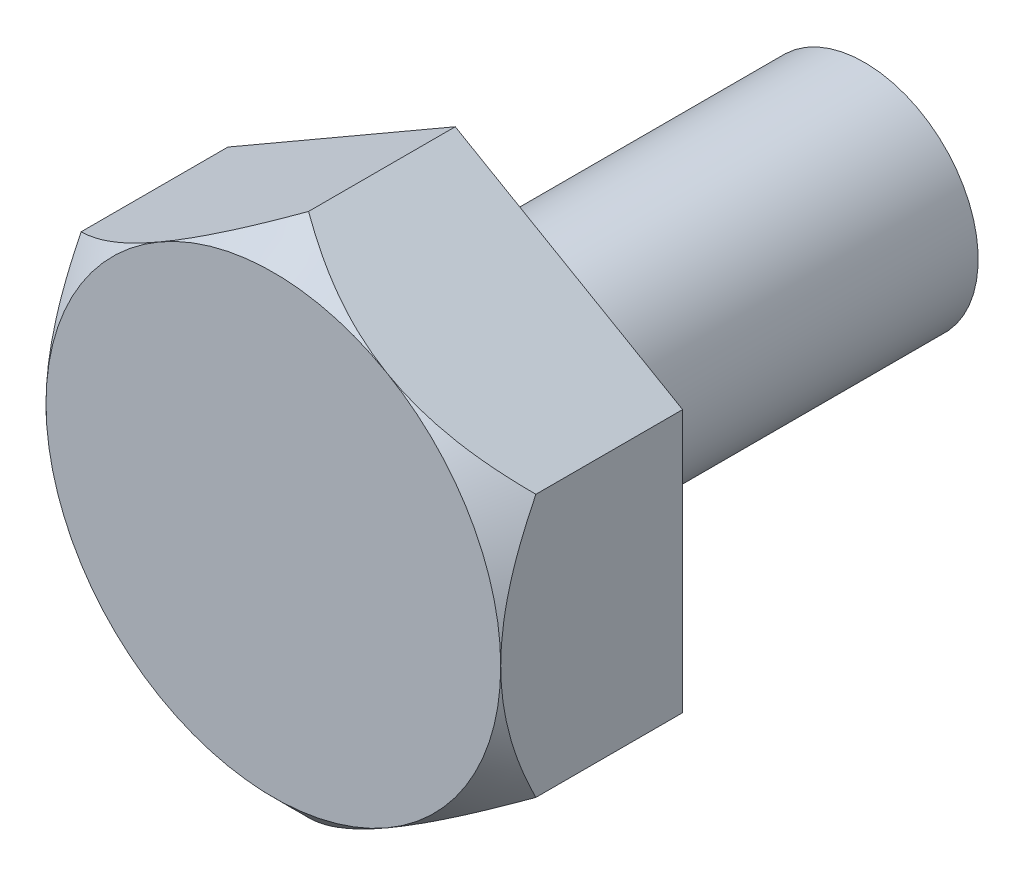
ISO-10303-21;
HEADER;
FILE_DESCRIPTION(('STEP AP214'),'2;1');
FILE_NAME('part.step','',(''),(''),'','','');
FILE_SCHEMA(('AUTOMOTIVE_DESIGN { 1 0 10303 214 1 1 1 1 }'));
ENDSEC;
DATA;
#1=APPLICATION_CONTEXT('core data for automotive mechanical design processes');
#2=APPLICATION_PROTOCOL_DEFINITION('international standard','automotive_design',2000,#1);
#3=PRODUCT_CONTEXT('',#1,'mechanical');
#4=PRODUCT('Part','Part','',(#3));
#5=PRODUCT_RELATED_PRODUCT_CATEGORY('part','',(#4));
#6=PRODUCT_DEFINITION_FORMATION('','',#4);
#7=PRODUCT_DEFINITION_CONTEXT('part definition',#1,'design');
#8=PRODUCT_DEFINITION('design','',#6,#7);
#9=PRODUCT_DEFINITION_SHAPE('','',#8);
#10=(LENGTH_UNIT() NAMED_UNIT(*) SI_UNIT(.MILLI.,.METRE.));
#11=(NAMED_UNIT(*) PLANE_ANGLE_UNIT() SI_UNIT($,.RADIAN.));
#12=(NAMED_UNIT(*) SI_UNIT($,.STERADIAN.) SOLID_ANGLE_UNIT());
#13=UNCERTAINTY_MEASURE_WITH_UNIT(LENGTH_MEASURE(1.E-05),#10,'distance_accuracy_value','');
#14=(GEOMETRIC_REPRESENTATION_CONTEXT(3) GLOBAL_UNCERTAINTY_ASSIGNED_CONTEXT((#13)) GLOBAL_UNIT_ASSIGNED_CONTEXT((#10,
#11,#12)) REPRESENTATION_CONTEXT('',''));
#15=CARTESIAN_POINT('',(0.,0.,0.));
#16=DIRECTION('',(0.,0.,1.));
#17=DIRECTION('',(1.,0.,0.));
#18=AXIS2_PLACEMENT_3D('',#15,#16,#17);
#19=CARTESIAN_POINT('',(0.,-5.77350269189626,4.));
#20=DIRECTION('',(-0.5,0.866025403784439,0.));
#21=DIRECTION('',(-0.866025403784439,-0.5,0.));
#22=AXIS2_PLACEMENT_3D('',#19,#20,#21);
#23=PLANE('',#22);
#24=CARTESIAN_POINT('',(-0.000200000000000018,-5.7736181619501,3.22638183458588));
#25=CARTESIAN_POINT('',(0.0857727681733069,-5.72398176110226,3.27601376249949));
#26=CARTESIAN_POINT('',(0.172406369471809,-5.67396382807171,3.32412258281684));
#27=CARTESIAN_POINT('',(0.347124889028839,-5.57309004377304,3.41683067677397));
#28=CARTESIAN_POINT('',(0.43521056864361,-5.5222337529357,3.46142803360226));
#29=CARTESIAN_POINT('',(0.702658569860331,-5.367822577439,3.58963823597549));
#30=CARTESIAN_POINT('',(0.884284999421829,-5.26296050943972,3.66712224260222));
#31=CARTESIAN_POINT('',(1.25054924277182,-5.05149774994707,3.79980836367823));
#32=CARTESIAN_POINT('',(1.43509343762461,-4.94495110937143,3.85534476745791));
#33=CARTESIAN_POINT('',(1.71494377217238,-4.78337944338747,3.91958681405623));
#34=CARTESIAN_POINT('',(1.8086392399128,-4.72928433986568,3.93781514476511));
#35=CARTESIAN_POINT('',(1.99682352572353,-4.6206360917956,3.96750512097762));
#36=CARTESIAN_POINT('',(2.09131222308105,-4.56608301694086,3.97896777779866));
#37=CARTESIAN_POINT('',(2.32156625980078,-4.43314578685873,3.99818644635776));
#38=CARTESIAN_POINT('',(2.45757968486243,-4.35461839928598,4.00221901984403));
#39=CARTESIAN_POINT('',(2.7293614118944,-4.19770514602325,3.99545145399843));
#40=CARTESIAN_POINT('',(2.86512961123582,-4.11931933958609,3.98464611513274));
#41=CARTESIAN_POINT('',(3.13538603207476,-3.96328672226451,3.9488396582057));
#42=CARTESIAN_POINT('',(3.26987265077585,-3.88564083675503,3.92382266414548));
#43=CARTESIAN_POINT('',(3.53653439939647,-3.73168360440634,3.86095298311431));
#44=CARTESIAN_POINT('',(3.66870970573537,-3.65537215571135,3.82310128033618));
#45=CARTESIAN_POINT('',(3.90334820652232,-3.51990355411976,3.7452274213432));
#46=CARTESIAN_POINT('',(4.0063308906988,-3.4604464736886,3.70725305768472));
#47=CARTESIAN_POINT('',(4.21044753419218,-3.34259967462161,3.62518468192979));
#48=CARTESIAN_POINT('',(4.31158143726392,-3.28420998845894,3.58109048400019));
#49=CARTESIAN_POINT('',(4.51168198823798,-3.16868188148908,3.48777092275138));
#50=CARTESIAN_POINT('',(4.61065432718709,-3.11154017495448,3.43856169539435));
#51=CARTESIAN_POINT('',(4.80676624461305,-2.99831490663731,3.33565818526074));
#52=CARTESIAN_POINT('',(4.90390690306938,-2.94223072132829,3.28196665355472));
#53=CARTESIAN_POINT('',(5.0002,-2.88663587589429,3.22638183458587));
#54=B_SPLINE_CURVE_WITH_KNOTS('',3,(#24,#25,#26,#27,#28,#29,#30,#31,#32,#33,#34,#35,#36,#37,#38,
#39,#40,#41,#42,#43,#44,#45,#46,#47,#48,#49,#50,#51,#52,#53),.UNSPECIFIED.,.F.,.F.,(4,2,2,2,2,2,
2,2,2,2,2,2,2,2,4),(0.,0.332945616209568,0.666071736106991,1.33592065243334,1.99513262597481,
2.32409207808824,2.65300234563691,3.12358963991983,3.59434188052354,4.06562104077027,
4.53686407049611,4.91117956742317,5.2855064331967,5.65868635377115,6.03163889109472),.UNSPECIFIED.);
#55=CARTESIAN_POINT('',(0.,-5.77350269189626,3.22649730810375));
#56=VERTEX_POINT('',#55);
#57=CARTESIAN_POINT('',(2.5,-4.3301270189222,4.));
#58=VERTEX_POINT('',#57);
#59=EDGE_CURVE('E225',#56,#58,#54,.T.);
#60=ORIENTED_EDGE('',*,*,#59,.F.);
#61=DIRECTION('',(0.,0.,-1.));
#62=VECTOR('',#61,1.);
#63=CARTESIAN_POINT('',(0.,-5.77350269189626,4.));
#64=LINE('',#63,#62);
#65=CARTESIAN_POINT('',(0.,-5.77350269189626,0.));
#66=VERTEX_POINT('',#65);
#67=EDGE_CURVE('E223',#56,#66,#64,.T.);
#68=ORIENTED_EDGE('',*,*,#67,.T.);
#69=DIRECTION('',(0.866025403784439,0.5,0.));
#70=VECTOR('',#69,1.);
#71=CARTESIAN_POINT('',(0.,-5.77350269189626,0.));
#72=LINE('',#71,#70);
#73=CARTESIAN_POINT('',(5.,-2.88675134594813,0.));
#74=VERTEX_POINT('',#73);
#75=EDGE_CURVE('E229',#66,#74,#72,.T.);
#76=ORIENTED_EDGE('',*,*,#75,.T.);
#77=DIRECTION('',(0.,0.,-1.));
#78=VECTOR('',#77,1.);
#79=CARTESIAN_POINT('',(5.,-2.88675134594813,4.));
#80=LINE('',#79,#78);
#81=CARTESIAN_POINT('',(5.,-2.88675134594815,3.22649730810375));
#82=VERTEX_POINT('',#81);
#83=EDGE_CURVE('E246',#82,#74,#80,.T.);
#84=ORIENTED_EDGE('',*,*,#83,.F.);
#85=EDGE_CURVE('E180',#58,#82,#54,.T.);
#86=ORIENTED_EDGE('',*,*,#85,.F.);
#87=EDGE_LOOP('',(#60,#68,#76,#84,#86));
#88=FACE_BOUND('',#87,.T.);
#89=ADVANCED_FACE('F45',(#88),#23,.F.);
#90=CARTESIAN_POINT('',(5.,-2.88675134594813,4.));
#91=DIRECTION('',(-1.,0.,0.));
#92=DIRECTION('',(0.,-1.,0.));
#93=AXIS2_PLACEMENT_3D('',#90,#91,#92);
#94=PLANE('',#93);
#95=CARTESIAN_POINT('',(5.,-9.91072051451662,-2.10055769395665));
#96=CARTESIAN_POINT('',(5.,-9.76621544127602,-1.97154454329479));
#97=CARTESIAN_POINT('',(5.,-9.62142904059379,-1.84284651390385));
#98=CARTESIAN_POINT('',(5.,-9.33121648801016,-1.58617055483695));
#99=CARTESIAN_POINT('',(5.,-9.18579032871603,-1.45819263352135));
#100=CARTESIAN_POINT('',(5.,-8.74834130441583,-1.07539053167285));
#101=CARTESIAN_POINT('',(5.,-8.45524720366472,-0.821786895816466));
#102=CARTESIAN_POINT('',(5.,-7.86187287101059,-0.315830598049089));
#103=CARTESIAN_POINT('',(5.,-7.56154861188113,-0.0635294286387808));
#104=CARTESIAN_POINT('',(5.,-6.95607062007869,0.435107261094935));
#105=CARTESIAN_POINT('',(5.,-6.65091784334251,0.681443938411082));
#106=CARTESIAN_POINT('',(5.,-6.05281956409636,1.15115601537285));
#107=CARTESIAN_POINT('',(5.,-5.76025864959821,1.37501719326704));
#108=CARTESIAN_POINT('',(5.,-5.3155611070372,1.70306559777502));
#109=CARTESIAN_POINT('',(5.,-5.1663052656364,1.81115689472442));
#110=CARTESIAN_POINT('',(5.,-4.86554936597768,2.02416494614329));
#111=CARTESIAN_POINT('',(5.,-4.71404941939871,2.12908185780219));
#112=CARTESIAN_POINT('',(5.,-4.40884314645316,2.33477509223266));
#113=CARTESIAN_POINT('',(5.,-4.25514378185362,2.43556171139529));
#114=CARTESIAN_POINT('',(5.,-3.94471151466891,2.63239951344171));
#115=CARTESIAN_POINT('',(5.,-3.78797837092588,2.72845031770066));
#116=CARTESIAN_POINT('',(5.,-3.47117914660732,2.91455296566001));
#117=CARTESIAN_POINT('',(5.,-3.31111650469861,3.00461063098044));
#118=CARTESIAN_POINT('',(5.,-2.98705558910371,3.17731119527027));
#119=CARTESIAN_POINT('',(5.,-2.82305823727669,3.25995580994437));
#120=CARTESIAN_POINT('',(5.,-2.50246960746522,3.41038679829273));
#121=CARTESIAN_POINT('',(5.,-2.34618024242307,3.47881169830795));
#122=CARTESIAN_POINT('',(5.,-2.02957491141866,3.60572985215042));
#123=CARTESIAN_POINT('',(5.,-1.86925893812462,3.66422308789225));
#124=CARTESIAN_POINT('',(5.,-1.54540593636024,3.76885041954304));
#125=CARTESIAN_POINT('',(5.,-1.38188714698498,3.81504020516505));
#126=CARTESIAN_POINT('',(5.,-1.05149027309675,3.89315112780065));
#127=CARTESIAN_POINT('',(5.,-0.884613565388637,3.9250779931138));
#128=CARTESIAN_POINT('',(5.,-0.545836980273731,3.97313093477257));
#129=CARTESIAN_POINT('',(5.,-0.373899433698271,3.98899706157323));
#130=CARTESIAN_POINT('',(5.,-0.0293097036115672,4.00287735940177));
#131=CARTESIAN_POINT('',(5.,0.143342399655701,4.00089348335961));
#132=CARTESIAN_POINT('',(5.,0.487882402140031,3.97920409445634));
#133=CARTESIAN_POINT('',(5.,0.659767847142363,3.95946033548157));
#134=CARTESIAN_POINT('',(5.,1.00084509884113,3.90359558221986));
#135=CARTESIAN_POINT('',(5.,1.17003611690969,3.86746988111293));
#136=CARTESIAN_POINT('',(5.,1.55360689626622,3.7683614441394));
#137=CARTESIAN_POINT('',(5.,1.76674581305401,3.70061559776904));
#138=CARTESIAN_POINT('',(5.,2.18611598773547,3.54647241114183));
#139=CARTESIAN_POINT('',(5.,2.39234343170509,3.4600649625223));
#140=CARTESIAN_POINT('',(5.,2.80040314281745,3.27207752711923));
#141=CARTESIAN_POINT('',(5.,3.00216331747143,3.17034289977823));
#142=CARTESIAN_POINT('',(5.,3.30029802660671,3.00959150256192));
#143=CARTESIAN_POINT('',(5.,3.39891511024584,2.9546557234027));
#144=CARTESIAN_POINT('',(5.,3.59478493952169,2.84240035369005));
#145=CARTESIAN_POINT('',(5.,3.69203769266294,2.78508077625563));
#146=CARTESIAN_POINT('',(5.,3.93268621485032,2.63974614813006));
#147=CARTESIAN_POINT('',(5.,4.07531703883476,2.55046551491085));
#148=CARTESIAN_POINT('',(5.,4.35814665684457,2.36812363187614));
#149=CARTESIAN_POINT('',(5.,4.49834523281012,2.27506204555858));
#150=CARTESIAN_POINT('',(5.,4.91585745402423,1.9911616420883));
#151=CARTESIAN_POINT('',(5.,5.19000092006772,1.79566062403075));
#152=CARTESIAN_POINT('',(5.,5.7323797860828,1.39561219564106));
#153=CARTESIAN_POINT('',(5.,6.00060231013792,1.19104751794871));
#154=CARTESIAN_POINT('',(5.,6.53211217027,0.775583147109073));
#155=CARTESIAN_POINT('',(5.,6.79539913149934,0.564682975932098));
#156=CARTESIAN_POINT('',(5.,7.30031300079127,0.15269603485646));
#157=CARTESIAN_POINT('',(5.,7.542193814675,-0.0480807930482146));
#158=CARTESIAN_POINT('',(5.,8.02327968337917,-0.452837162951994));
#159=CARTESIAN_POINT('',(5.,8.26248458717145,-0.656816884175983));
#160=CARTESIAN_POINT('',(5.,8.73754753272066,-1.06629372433063));
#161=CARTESIAN_POINT('',(5.,8.97341623310163,-1.27177850235316));
#162=CARTESIAN_POINT('',(5.,9.44333428124391,-1.68476461510824));
#163=CARTESIAN_POINT('',(5.,9.67738383656504,-1.89226571351926));
#164=CARTESIAN_POINT('',(5.,9.91072051451663,-2.10055769395665));
#165=B_SPLINE_CURVE_WITH_KNOTS('',3,(#95,#96,#97,#98,#99,#100,#101,#102,#103,#104,#105,#106,
#107,#108,#109,#110,#111,#112,#113,#114,#115,#116,#117,#118,#119,#120,#121,#122,#123,#124,#125,
#126,#127,#128,#129,#130,#131,#132,#133,#134,#135,#136,#137,#138,#139,#140,#141,#142,#143,#144,
#145,#146,#147,#148,#149,#150,#151,#152,#153,#154,#155,#156,#157,#158,#159,#160,#161,#162,#163,
#164),.UNSPECIFIED.,.F.,.F.,(4,2,2,2,2,2,2,2,2,2,2,2,2,2,2,2,2,2,2,2,2,2,2,2,2,2,2,2,2,2,2,2,2,
2,4),(0.,0.581148909212411,1.16230455163196,2.32501564731192,3.50167323602094,4.67810071770477,
5.78306048880437,6.33588410810416,6.88868030769224,7.44000224568793,7.99136819022149,
8.5421904855475,9.09288496573265,9.6044443239522,10.1160046137044,10.6252084636211,
11.1342076219167,11.6513194059097,12.1683746145159,12.6865459803083,13.2048663202667,
13.8746333370564,14.5447640581128,15.2221753046931,15.5608090570693,15.8994409460531,
16.4041719839859,16.9089480414397,17.9188053190632,18.9306770062131,19.9426252344689,
20.8856511270215,21.8287299780402,22.7671855689286,23.7055324644857),.UNSPECIFIED.);
#166=CARTESIAN_POINT('',(5.,0.,4.));
#167=VERTEX_POINT('',#166);
#168=EDGE_CURVE('E271',#82,#167,#165,.T.);
#169=ORIENTED_EDGE('',*,*,#168,.F.);
#170=ORIENTED_EDGE('',*,*,#83,.T.);
#171=DIRECTION('',(0.,1.,0.));
#172=VECTOR('',#171,1.);
#173=CARTESIAN_POINT('',(5.,-2.88675134594813,0.));
#174=LINE('',#173,#172);
#175=CARTESIAN_POINT('',(5.,2.88675134594813,0.));
#176=VERTEX_POINT('',#175);
#177=EDGE_CURVE('E266',#74,#176,#174,.T.);
#178=ORIENTED_EDGE('',*,*,#177,.T.);
#179=DIRECTION('',(0.,0.,-1.));
#180=VECTOR('',#179,1.);
#181=CARTESIAN_POINT('',(5.,2.88675134594813,4.));
#182=LINE('',#181,#180);
#183=CARTESIAN_POINT('',(5.,2.88675134594813,3.22649730810375));
#184=VERTEX_POINT('',#183);
#185=EDGE_CURVE('E245',#184,#176,#182,.T.);
#186=ORIENTED_EDGE('',*,*,#185,.F.);
#187=EDGE_CURVE('E118',#167,#184,#165,.T.);
#188=ORIENTED_EDGE('',*,*,#187,.F.);
#189=EDGE_LOOP('',(#169,#170,#178,#186,#188));
#190=FACE_BOUND('',#189,.T.);
#191=ADVANCED_FACE('F213',(#190),#94,.F.);
#192=CARTESIAN_POINT('',(5.,2.88675134594813,4.));
#193=DIRECTION('',(-0.5,-0.866025403784439,0.));
#194=DIRECTION('',(0.866025403784439,-0.5,0.));
#195=AXIS2_PLACEMENT_3D('',#192,#193,#194);
#196=PLANE('',#195);
#197=CARTESIAN_POINT('',(5.0002,2.88663587589429,3.22638183458588));
#198=CARTESIAN_POINT('',(4.91422723182669,2.93627227674213,3.27601376249948));
#199=CARTESIAN_POINT('',(4.82759363052819,2.98629020977269,3.32412258281684));
#200=CARTESIAN_POINT('',(4.65287511097116,3.08716399407135,3.41683067677397));
#201=CARTESIAN_POINT('',(4.56478943135639,3.13802028490869,3.46142803360226));
#202=CARTESIAN_POINT('',(4.29734143013967,3.29243146040539,3.58963823597549));
#203=CARTESIAN_POINT('',(4.11571500057817,3.39729352840467,3.66712224260222));
#204=CARTESIAN_POINT('',(3.74945075722818,3.60875628789733,3.79980836367823));
#205=CARTESIAN_POINT('',(3.56490656237539,3.71530292847296,3.85534476745791));
#206=CARTESIAN_POINT('',(3.28505622782762,3.87687459445692,3.91958681405623));
#207=CARTESIAN_POINT('',(3.1913607600872,3.93096969797871,3.93781514476511));
#208=CARTESIAN_POINT('',(3.00317647427647,4.03961794604879,3.96750512097762));
#209=CARTESIAN_POINT('',(2.90868777691895,4.09417102090353,3.97896777779866));
#210=CARTESIAN_POINT('',(2.67843374019922,4.22710825098566,3.99818644635776));
#211=CARTESIAN_POINT('',(2.54242031513757,4.30563563855841,4.00221901984403));
#212=CARTESIAN_POINT('',(2.2706385881056,4.46254889182114,3.99545145399843));
#213=CARTESIAN_POINT('',(2.13487038876418,4.5409346982583,3.98464611513274));
#214=CARTESIAN_POINT('',(1.86461396792524,4.69696731557988,3.9488396582057));
#215=CARTESIAN_POINT('',(1.73012734922416,4.77461320108936,3.92382266414548));
#216=CARTESIAN_POINT('',(1.46346560060354,4.92857043343805,3.86095298311431));
#217=CARTESIAN_POINT('',(1.33129029426463,5.00488188213304,3.82310128033618));
#218=CARTESIAN_POINT('',(1.09665179347769,5.14035048372463,3.7452274213432));
#219=CARTESIAN_POINT('',(0.993669109301204,5.19980756415579,3.70725305768472));
#220=CARTESIAN_POINT('',(0.789552465807829,5.31765436322278,3.62518468192979));
#221=CARTESIAN_POINT('',(0.688418562736081,5.37604404938545,3.58109048400019));
#222=CARTESIAN_POINT('',(0.488318011762026,5.49157215635531,3.48777092275138));
#223=CARTESIAN_POINT('',(0.38934567281291,5.54871386288991,3.43856169539435));
#224=CARTESIAN_POINT('',(0.193233755386958,5.66193913120708,3.33565818526074));
#225=CARTESIAN_POINT('',(0.0960930969306188,5.7180233165161,3.28196665355472));
#226=CARTESIAN_POINT('',(-0.000199999999999045,5.7736181619501,3.22638183458588));
#227=B_SPLINE_CURVE_WITH_KNOTS('',3,(#197,#198,#199,#200,#201,#202,#203,#204,#205,#206,#207,
#208,#209,#210,#211,#212,#213,#214,#215,#216,#217,#218,#219,#220,#221,#222,#223,#224,#225,#226),
.UNSPECIFIED.,.F.,.F.,(4,2,2,2,2,2,2,2,2,2,2,2,2,2,4),(0.,0.332945616209569,0.666071736106991,
1.33592065243334,1.99513262597481,2.32409207808824,2.65300234563691,3.12358963991983,
3.59434188052354,4.06562104077027,4.53686407049611,4.91117956742317,5.2855064331967,
5.65868635377115,6.03163889109472),.UNSPECIFIED.);
#228=CARTESIAN_POINT('',(2.5,4.3301270189222,4.));
#229=VERTEX_POINT('',#228);
#230=EDGE_CURVE('E113',#184,#229,#227,.T.);
#231=ORIENTED_EDGE('',*,*,#230,.F.);
#232=ORIENTED_EDGE('',*,*,#185,.T.);
#233=DIRECTION('',(-0.866025403784439,0.5,0.));
#234=VECTOR('',#233,1.);
#235=CARTESIAN_POINT('',(5.,2.88675134594813,0.));
#236=LINE('',#235,#234);
#237=CARTESIAN_POINT('',(0.,5.77350269189626,0.));
#238=VERTEX_POINT('',#237);
#239=EDGE_CURVE('E270',#176,#238,#236,.T.);
#240=ORIENTED_EDGE('',*,*,#239,.T.);
#241=DIRECTION('',(0.,0.,-1.));
#242=VECTOR('',#241,1.);
#243=CARTESIAN_POINT('',(0.,5.77350269189626,4.));
#244=LINE('',#243,#242);
#245=CARTESIAN_POINT('',(0.,5.77350269189626,3.22649730810375));
#246=VERTEX_POINT('',#245);
#247=EDGE_CURVE('E142',#246,#238,#244,.T.);
#248=ORIENTED_EDGE('',*,*,#247,.F.);
#249=EDGE_CURVE('E122',#229,#246,#227,.T.);
#250=ORIENTED_EDGE('',*,*,#249,.F.);
#251=EDGE_LOOP('',(#231,#232,#240,#248,#250));
#252=FACE_BOUND('',#251,.T.);
#253=ADVANCED_FACE('F139',(#252),#196,.F.);
#254=CARTESIAN_POINT('',(0.,5.77350269189626,4.));
#255=DIRECTION('',(0.5,-0.866025403784439,0.));
#256=DIRECTION('',(0.866025403784439,0.5,0.));
#257=AXIS2_PLACEMENT_3D('',#254,#255,#256);
#258=PLANE('',#257);
#259=CARTESIAN_POINT('',(0.000200000000001333,5.7736181619501,3.22638183458588));
#260=CARTESIAN_POINT('',(-0.085772768173306,5.72398176110226,3.27601376249948));
#261=CARTESIAN_POINT('',(-0.172406369471808,5.67396382807171,3.32412258281684));
#262=CARTESIAN_POINT('',(-0.347124889028838,5.57309004377304,3.41683067677397));
#263=CARTESIAN_POINT('',(-0.435210568643609,5.5222337529357,3.46142803360226));
#264=CARTESIAN_POINT('',(-0.70265856986033,5.367822577439,3.58963823597549));
#265=CARTESIAN_POINT('',(-0.884284999421829,5.26296050943972,3.66712224260222));
#266=CARTESIAN_POINT('',(-1.25054924277182,5.05149774994706,3.79980836367823));
#267=CARTESIAN_POINT('',(-1.43509343762461,4.94495110937143,3.85534476745791));
#268=CARTESIAN_POINT('',(-1.71494377217238,4.78337944338747,3.91958681405623));
#269=CARTESIAN_POINT('',(-1.8086392399128,4.72928433986569,3.93781514476511));
#270=CARTESIAN_POINT('',(-1.99682352572353,4.6206360917956,3.96750512097762));
#271=CARTESIAN_POINT('',(-2.09131222308105,4.56608301694086,3.97896777779866));
#272=CARTESIAN_POINT('',(-2.32156625980078,4.43314578685873,3.99818644635776));
#273=CARTESIAN_POINT('',(-2.45757968486243,4.35461839928598,4.00221901984403));
#274=CARTESIAN_POINT('',(-2.7293614118944,4.19770514602325,3.99545145399843));
#275=CARTESIAN_POINT('',(-2.86512961123582,4.11931933958609,3.98464611513274));
#276=CARTESIAN_POINT('',(-3.13538603207476,3.96328672226451,3.9488396582057));
#277=CARTESIAN_POINT('',(-3.26987265077584,3.88564083675503,3.92382266414548));
#278=CARTESIAN_POINT('',(-3.53653439939646,3.73168360440634,3.86095298311431));
#279=CARTESIAN_POINT('',(-3.66870970573537,3.65537215571135,3.82310128033618));
#280=CARTESIAN_POINT('',(-3.90334820652231,3.51990355411976,3.7452274213432));
#281=CARTESIAN_POINT('',(-4.0063308906988,3.4604464736886,3.70725305768472));
#282=CARTESIAN_POINT('',(-4.21044753419217,3.34259967462161,3.6251846819298));
#283=CARTESIAN_POINT('',(-4.31158143726392,3.28420998845894,3.58109048400019));
#284=CARTESIAN_POINT('',(-4.51168198823798,3.16868188148908,3.48777092275138));
#285=CARTESIAN_POINT('',(-4.61065432718709,3.11154017495448,3.43856169539435));
#286=CARTESIAN_POINT('',(-4.80676624461304,2.99831490663731,3.33565818526074));
#287=CARTESIAN_POINT('',(-4.90390690306938,2.94223072132829,3.28196665355473));
#288=CARTESIAN_POINT('',(-5.0002,2.88663587589429,3.22638183458588));
#289=B_SPLINE_CURVE_WITH_KNOTS('',3,(#259,#260,#261,#262,#263,#264,#265,#266,#267,#268,#269,
#270,#271,#272,#273,#274,#275,#276,#277,#278,#279,#280,#281,#282,#283,#284,#285,#286,#287,#288),
.UNSPECIFIED.,.F.,.F.,(4,2,2,2,2,2,2,2,2,2,2,2,2,2,4),(0.,0.332945616209568,0.666071736106991,
1.33592065243334,1.99513262597481,2.32409207808824,2.65300234563691,3.12358963991983,
3.59434188052353,4.06562104077027,4.53686407049611,4.91117956742317,5.2855064331967,
5.65868635377115,6.03163889109472),.UNSPECIFIED.);
#290=CARTESIAN_POINT('',(-2.5,4.3301270189222,4.));
#291=VERTEX_POINT('',#290);
#292=EDGE_CURVE('E129',#246,#291,#289,.T.);
#293=ORIENTED_EDGE('',*,*,#292,.F.);
#294=ORIENTED_EDGE('',*,*,#247,.T.);
#295=DIRECTION('',(-0.866025403784439,-0.5,0.));
#296=VECTOR('',#295,1.);
#297=CARTESIAN_POINT('',(0.,5.77350269189626,0.));
#298=LINE('',#297,#296);
#299=CARTESIAN_POINT('',(-5.,2.88675134594813,0.));
#300=VERTEX_POINT('',#299);
#301=EDGE_CURVE('E263',#238,#300,#298,.T.);
#302=ORIENTED_EDGE('',*,*,#301,.T.);
#303=DIRECTION('',(0.,0.,-1.));
#304=VECTOR('',#303,1.);
#305=CARTESIAN_POINT('',(-5.,2.88675134594813,4.));
#306=LINE('',#305,#304);
#307=CARTESIAN_POINT('',(-5.,2.88675134594815,3.22649730810375));
#308=VERTEX_POINT('',#307);
#309=EDGE_CURVE('E240',#308,#300,#306,.T.);
#310=ORIENTED_EDGE('',*,*,#309,.F.);
#311=EDGE_CURVE('E141',#291,#308,#289,.T.);
#312=ORIENTED_EDGE('',*,*,#311,.F.);
#313=EDGE_LOOP('',(#293,#294,#302,#310,#312));
#314=FACE_BOUND('',#313,.T.);
#315=ADVANCED_FACE('F204',(#314),#258,.F.);
#316=CARTESIAN_POINT('',(-5.,2.88675134594813,4.));
#317=DIRECTION('',(1.,0.,0.));
#318=DIRECTION('',(0.,0.,-1.));
#319=AXIS2_PLACEMENT_3D('',#316,#317,#318);
#320=PLANE('',#319);
#321=CARTESIAN_POINT('',(-5.,9.91072051451663,-2.10055769395665));
#322=CARTESIAN_POINT('',(-5.,9.76621544127602,-1.97154454329479));
#323=CARTESIAN_POINT('',(-5.,9.62142904059379,-1.84284651390385));
#324=CARTESIAN_POINT('',(-5.,9.33121648801016,-1.58617055483695));
#325=CARTESIAN_POINT('',(-5.,9.18579032871603,-1.45819263352135));
#326=CARTESIAN_POINT('',(-5.,8.74834130441583,-1.07539053167285));
#327=CARTESIAN_POINT('',(-5.,8.45524720366472,-0.821786895816467));
#328=CARTESIAN_POINT('',(-5.,7.86187287101059,-0.315830598049089));
#329=CARTESIAN_POINT('',(-5.,7.56154861188114,-0.0635294286387806));
#330=CARTESIAN_POINT('',(-5.,6.95607062007869,0.435107261094936));
#331=CARTESIAN_POINT('',(-5.,6.65091784334251,0.681443938411084));
#332=CARTESIAN_POINT('',(-5.,6.05281956409636,1.15115601537285));
#333=CARTESIAN_POINT('',(-5.,5.76025864959822,1.37501719326704));
#334=CARTESIAN_POINT('',(-5.,5.3155611070372,1.70306559777502));
#335=CARTESIAN_POINT('',(-5.,5.1663052656364,1.81115689472442));
#336=CARTESIAN_POINT('',(-5.,4.86554936597768,2.02416494614329));
#337=CARTESIAN_POINT('',(-5.,4.71404941939871,2.12908185780219));
#338=CARTESIAN_POINT('',(-5.,4.40884314645316,2.33477509223266));
#339=CARTESIAN_POINT('',(-5.,4.25514378185362,2.43556171139529));
#340=CARTESIAN_POINT('',(-5.,3.94471151466891,2.63239951344171));
#341=CARTESIAN_POINT('',(-5.,3.78797837092588,2.72845031770066));
#342=CARTESIAN_POINT('',(-5.,3.47117914660733,2.91455296566001));
#343=CARTESIAN_POINT('',(-5.,3.31111650469862,3.00461063098044));
#344=CARTESIAN_POINT('',(-5.,2.98705558910371,3.17731119527027));
#345=CARTESIAN_POINT('',(-5.,2.82305823727669,3.25995580994437));
#346=CARTESIAN_POINT('',(-5.,2.50246960746522,3.41038679829273));
#347=CARTESIAN_POINT('',(-5.,2.34618024242307,3.47881169830795));
#348=CARTESIAN_POINT('',(-5.,2.02957491141867,3.60572985215042));
#349=CARTESIAN_POINT('',(-5.,1.86925893812462,3.66422308789225));
#350=CARTESIAN_POINT('',(-5.,1.54540593636025,3.76885041954304));
#351=CARTESIAN_POINT('',(-5.,1.38188714698499,3.81504020516505));
#352=CARTESIAN_POINT('',(-5.,1.05149027309676,3.89315112780065));
#353=CARTESIAN_POINT('',(-5.,0.884613565388641,3.9250779931138));
#354=CARTESIAN_POINT('',(-5.,0.545836980273738,3.97313093477257));
#355=CARTESIAN_POINT('',(-5.,0.373899433698277,3.98899706157323));
#356=CARTESIAN_POINT('',(-5.,0.0293097036115736,4.00287735940177));
#357=CARTESIAN_POINT('',(-5.,-0.143342399655695,4.00089348335961));
#358=CARTESIAN_POINT('',(-5.,-0.487882402140026,3.97920409445635));
#359=CARTESIAN_POINT('',(-5.,-0.659767847142358,3.95946033548157));
#360=CARTESIAN_POINT('',(-5.,-1.00084509884112,3.90359558221986));
#361=CARTESIAN_POINT('',(-5.,-1.17003611690968,3.86746988111293));
#362=CARTESIAN_POINT('',(-5.,-1.55360689626622,3.7683614441394));
#363=CARTESIAN_POINT('',(-5.,-1.76674581305401,3.70061559776904));
#364=CARTESIAN_POINT('',(-5.,-2.18611598773546,3.54647241114183));
#365=CARTESIAN_POINT('',(-5.,-2.39234343170509,3.4600649625223));
#366=CARTESIAN_POINT('',(-5.,-2.80040314281745,3.27207752711923));
#367=CARTESIAN_POINT('',(-5.,-3.00216331747142,3.17034289977824));
#368=CARTESIAN_POINT('',(-5.,-3.3002980266067,3.00959150256193));
#369=CARTESIAN_POINT('',(-5.,-3.39891511024583,2.95465572340271));
#370=CARTESIAN_POINT('',(-5.,-3.59478493952168,2.84240035369006));
#371=CARTESIAN_POINT('',(-5.,-3.69203769266292,2.78508077625564));
#372=CARTESIAN_POINT('',(-5.,-3.93268621485031,2.63974614813007));
#373=CARTESIAN_POINT('',(-5.,-4.07531703883475,2.55046551491086));
#374=CARTESIAN_POINT('',(-5.,-4.35814665684456,2.36812363187615));
#375=CARTESIAN_POINT('',(-5.,-4.49834523281012,2.27506204555858));
#376=CARTESIAN_POINT('',(-5.,-4.91585745402422,1.99116164208831));
#377=CARTESIAN_POINT('',(-5.,-5.19000092006771,1.79566062403075));
#378=CARTESIAN_POINT('',(-5.,-5.7323797860828,1.39561219564107));
#379=CARTESIAN_POINT('',(-5.,-6.00060231013791,1.19104751794872));
#380=CARTESIAN_POINT('',(-5.,-6.53211217027,0.775583147109079));
#381=CARTESIAN_POINT('',(-5.,-6.79539913149933,0.564682975932104));
#382=CARTESIAN_POINT('',(-5.,-7.30031300079127,0.152696034856465));
#383=CARTESIAN_POINT('',(-5.,-7.542193814675,-0.0480807930482094));
#384=CARTESIAN_POINT('',(-5.,-8.02327968337917,-0.452837162951989));
#385=CARTESIAN_POINT('',(-5.,-8.26248458717144,-0.65681688417598));
#386=CARTESIAN_POINT('',(-5.,-8.73754753272065,-1.06629372433062));
#387=CARTESIAN_POINT('',(-5.,-8.97341623310163,-1.27177850235316));
#388=CARTESIAN_POINT('',(-5.,-9.44333428124391,-1.68476461510824));
#389=CARTESIAN_POINT('',(-5.,-9.67738383656504,-1.89226571351926));
#390=CARTESIAN_POINT('',(-5.,-9.91072051451662,-2.10055769395665));
#391=B_SPLINE_CURVE_WITH_KNOTS('',3,(#321,#322,#323,#324,#325,#326,#327,#328,#329,#330,#331,
#332,#333,#334,#335,#336,#337,#338,#339,#340,#341,#342,#343,#344,#345,#346,#347,#348,#349,#350,
#351,#352,#353,#354,#355,#356,#357,#358,#359,#360,#361,#362,#363,#364,#365,#366,#367,#368,#369,
#370,#371,#372,#373,#374,#375,#376,#377,#378,#379,#380,#381,#382,#383,#384,#385,#386,#387,#388,
#389,#390),.UNSPECIFIED.,.F.,.F.,(4,2,2,2,2,2,2,2,2,2,2,2,2,2,2,2,2,2,2,2,2,2,2,2,2,2,2,2,2,2,2,
2,2,2,4),(0.,0.581148909212412,1.16230455163196,2.32501564731192,3.50167323602094,
4.67810071770477,5.78306048880437,6.33588410810416,6.88868030769224,7.44000224568794,
7.99136819022149,8.5421904855475,9.09288496573265,9.6044443239522,10.1160046137044,
10.6252084636211,11.1342076219167,11.6513194059097,12.1683746145159,12.6865459803083,
13.2048663202667,13.8746333370564,14.5447640581128,15.2221753046931,15.5608090570693,
15.8994409460531,16.4041719839859,16.9089480414397,17.9188053190632,18.9306770062131,
19.9426252344689,20.8856511270215,21.8287299780402,22.7671855689286,23.7055324644857),.UNSPECIFIED.);
#392=CARTESIAN_POINT('',(-5.,0.,4.));
#393=VERTEX_POINT('',#392);
#394=EDGE_CURVE('E196',#308,#393,#391,.T.);
#395=ORIENTED_EDGE('',*,*,#394,.F.);
#396=ORIENTED_EDGE('',*,*,#309,.T.);
#397=DIRECTION('',(0.,-1.,0.));
#398=VECTOR('',#397,1.);
#399=CARTESIAN_POINT('',(-5.,2.88675134594813,0.));
#400=LINE('',#399,#398);
#401=CARTESIAN_POINT('',(-5.,-2.88675134594813,0.));
#402=VERTEX_POINT('',#401);
#403=EDGE_CURVE('E239',#300,#402,#400,.T.);
#404=ORIENTED_EDGE('',*,*,#403,.T.);
#405=DIRECTION('',(0.,0.,-1.));
#406=VECTOR('',#405,1.);
#407=CARTESIAN_POINT('',(-5.,-2.88675134594813,4.));
#408=LINE('',#407,#406);
#409=CARTESIAN_POINT('',(-5.,-2.88675134594813,3.22649730810375));
#410=VERTEX_POINT('',#409);
#411=EDGE_CURVE('E234',#410,#402,#408,.T.);
#412=ORIENTED_EDGE('',*,*,#411,.F.);
#413=EDGE_CURVE('E195',#393,#410,#391,.T.);
#414=ORIENTED_EDGE('',*,*,#413,.F.);
#415=EDGE_LOOP('',(#395,#396,#404,#412,#414));
#416=FACE_BOUND('',#415,.T.);
#417=ADVANCED_FACE('F199',(#416),#320,.F.);
#418=CARTESIAN_POINT('',(-5.,-2.88675134594813,4.));
#419=DIRECTION('',(0.5,0.866025403784439,0.));
#420=DIRECTION('',(-0.866025403784439,0.5,0.));
#421=AXIS2_PLACEMENT_3D('',#418,#419,#420);
#422=PLANE('',#421);
#423=CARTESIAN_POINT('',(-5.0002,-2.88663587589429,3.22638183458588));
#424=CARTESIAN_POINT('',(-4.91422723182669,-2.93627227674213,3.27601376249949));
#425=CARTESIAN_POINT('',(-4.82759363052819,-2.98629020977269,3.32412258281684));
#426=CARTESIAN_POINT('',(-4.65287511097116,-3.08716399407135,3.41683067677397));
#427=CARTESIAN_POINT('',(-4.56478943135639,-3.13802028490869,3.46142803360226));
#428=CARTESIAN_POINT('',(-4.29734143013967,-3.29243146040539,3.58963823597549));
#429=CARTESIAN_POINT('',(-4.11571500057817,-3.39729352840467,3.66712224260222));
#430=CARTESIAN_POINT('',(-3.74945075722818,-3.60875628789732,3.79980836367823));
#431=CARTESIAN_POINT('',(-3.56490656237539,-3.71530292847296,3.85534476745791));
#432=CARTESIAN_POINT('',(-3.28505622782762,-3.87687459445692,3.91958681405623));
#433=CARTESIAN_POINT('',(-3.1913607600872,-3.93096969797871,3.93781514476511));
#434=CARTESIAN_POINT('',(-3.00317647427647,-4.03961794604879,3.96750512097762));
#435=CARTESIAN_POINT('',(-2.90868777691895,-4.09417102090353,3.97896777779866));
#436=CARTESIAN_POINT('',(-2.67843374019922,-4.22710825098566,3.99818644635776));
#437=CARTESIAN_POINT('',(-2.54242031513757,-4.30563563855841,4.00221901984403));
#438=CARTESIAN_POINT('',(-2.2706385881056,-4.46254889182114,3.99545145399843));
#439=CARTESIAN_POINT('',(-2.13487038876418,-4.5409346982583,3.98464611513274));
#440=CARTESIAN_POINT('',(-1.86461396792524,-4.69696731557988,3.9488396582057));
#441=CARTESIAN_POINT('',(-1.73012734922416,-4.77461320108936,3.92382266414548));
#442=CARTESIAN_POINT('',(-1.46346560060353,-4.92857043343805,3.86095298311431));
#443=CARTESIAN_POINT('',(-1.33129029426463,-5.00488188213304,3.82310128033618));
#444=CARTESIAN_POINT('',(-1.09665179347769,-5.14035048372463,3.7452274213432));
#445=CARTESIAN_POINT('',(-0.993669109301202,-5.19980756415579,3.70725305768472));
#446=CARTESIAN_POINT('',(-0.789552465807827,-5.31765436322278,3.6251846819298));
#447=CARTESIAN_POINT('',(-0.688418562736079,-5.37604404938545,3.58109048400019));
#448=CARTESIAN_POINT('',(-0.488318011762024,-5.49157215635531,3.48777092275138));
#449=CARTESIAN_POINT('',(-0.389345672812908,-5.54871386288991,3.43856169539435));
#450=CARTESIAN_POINT('',(-0.193233755386956,-5.66193913120708,3.33565818526074));
#451=CARTESIAN_POINT('',(-0.0960930969306174,-5.7180233165161,3.28196665355472));
#452=CARTESIAN_POINT('',(0.000200000000000515,-5.7736181619501,3.22638183458588));
#453=B_SPLINE_CURVE_WITH_KNOTS('',3,(#423,#424,#425,#426,#427,#428,#429,#430,#431,#432,#433,
#434,#435,#436,#437,#438,#439,#440,#441,#442,#443,#444,#445,#446,#447,#448,#449,#450,#451,#452),
.UNSPECIFIED.,.F.,.F.,(4,2,2,2,2,2,2,2,2,2,2,2,2,2,4),(0.,0.332945616209569,0.666071736106991,
1.33592065243334,1.99513262597481,2.32409207808824,2.65300234563691,3.12358963991983,
3.59434188052354,4.06562104077027,4.53686407049611,4.91117956742317,5.2855064331967,
5.65868635377115,6.03163889109472),.UNSPECIFIED.);
#454=CARTESIAN_POINT('',(-2.5,-4.33012701892219,4.));
#455=VERTEX_POINT('',#454);
#456=EDGE_CURVE('E200',#410,#455,#453,.T.);
#457=ORIENTED_EDGE('',*,*,#456,.F.);
#458=ORIENTED_EDGE('',*,*,#411,.T.);
#459=DIRECTION('',(0.866025403784439,-0.5,0.));
#460=VECTOR('',#459,1.);
#461=CARTESIAN_POINT('',(-5.,-2.88675134594813,0.));
#462=LINE('',#461,#460);
#463=EDGE_CURVE('E232',#402,#66,#462,.T.);
#464=ORIENTED_EDGE('',*,*,#463,.T.);
#465=ORIENTED_EDGE('',*,*,#67,.F.);
#466=EDGE_CURVE('E136',#455,#56,#453,.T.);
#467=ORIENTED_EDGE('',*,*,#466,.F.);
#468=EDGE_LOOP('',(#457,#458,#464,#465,#467));
#469=FACE_BOUND('',#468,.T.);
#470=ADVANCED_FACE('F201',(#469),#422,.F.);
#471=CARTESIAN_POINT('',(0.,0.,0.));
#472=DIRECTION('',(0.,0.,1.));
#473=DIRECTION('',(1.,0.,0.));
#474=AXIS2_PLACEMENT_3D('',#471,#472,#473);
#475=PLANE('',#474);
#476=CARTESIAN_POINT('',(0.,0.,0.));
#477=DIRECTION('',(0.,0.,-1.));
#478=DIRECTION('',(-1.,0.,0.));
#479=AXIS2_PLACEMENT_3D('',#476,#477,#478);
#480=CIRCLE('',#479,2.5);
#481=CARTESIAN_POINT('',(-2.5,0.,0.));
#482=VERTEX_POINT('',#481);
#483=EDGE_CURVE('E12',#482,#482,#480,.T.);
#484=ORIENTED_EDGE('',*,*,#483,.F.);
#485=EDGE_LOOP('',(#484));
#486=FACE_BOUND('',#485,.T.);
#487=ORIENTED_EDGE('',*,*,#75,.F.);
#488=ORIENTED_EDGE('',*,*,#463,.F.);
#489=ORIENTED_EDGE('',*,*,#403,.F.);
#490=ORIENTED_EDGE('',*,*,#301,.F.);
#491=ORIENTED_EDGE('',*,*,#239,.F.);
#492=ORIENTED_EDGE('',*,*,#177,.F.);
#493=EDGE_LOOP('',(#487,#488,#489,#490,#491,#492));
#494=FACE_BOUND('',#493,.T.);
#495=ADVANCED_FACE('F262',(#486,#494),#475,.F.);
#496=CARTESIAN_POINT('',(0.,0.,4.));
#497=DIRECTION('',(0.,0.,-1.));
#498=DIRECTION('',(1.,0.,0.));
#499=AXIS2_PLACEMENT_3D('',#496,#497,#498);
#500=CONICAL_SURFACE('',#499,5.,0.78539816339745);
#501=ORIENTED_EDGE('',*,*,#85,.T.);
#502=ORIENTED_EDGE('',*,*,#168,.T.);
#503=CARTESIAN_POINT('',(0.,0.,4.));
#504=DIRECTION('',(0.,0.,1.));
#505=DIRECTION('',(1.,0.,0.));
#506=AXIS2_PLACEMENT_3D('',#503,#504,#505);
#507=CIRCLE('',#506,5.);
#508=EDGE_CURVE('E46',#58,#167,#507,.T.);
#509=ORIENTED_EDGE('',*,*,#508,.F.);
#510=EDGE_LOOP('',(#501,#502,#509));
#511=FACE_BOUND('',#510,.T.);
#512=ADVANCED_FACE('F168',(#511),#500,.T.);
#513=ORIENTED_EDGE('',*,*,#59,.T.);
#514=EDGE_CURVE('E249',#455,#58,#507,.T.);
#515=ORIENTED_EDGE('',*,*,#514,.F.);
#516=ORIENTED_EDGE('',*,*,#466,.T.);
#517=EDGE_LOOP('',(#513,#515,#516));
#518=FACE_BOUND('',#517,.T.);
#519=ADVANCED_FACE('F163',(#518),#500,.T.);
#520=ORIENTED_EDGE('',*,*,#413,.T.);
#521=ORIENTED_EDGE('',*,*,#456,.T.);
#522=EDGE_CURVE('E70',#393,#455,#507,.T.);
#523=ORIENTED_EDGE('',*,*,#522,.F.);
#524=EDGE_LOOP('',(#520,#521,#523));
#525=FACE_BOUND('',#524,.T.);
#526=ADVANCED_FACE('F166',(#525),#500,.T.);
#527=ORIENTED_EDGE('',*,*,#311,.T.);
#528=ORIENTED_EDGE('',*,*,#394,.T.);
#529=EDGE_CURVE('E132',#291,#393,#507,.T.);
#530=ORIENTED_EDGE('',*,*,#529,.F.);
#531=EDGE_LOOP('',(#527,#528,#530));
#532=FACE_BOUND('',#531,.T.);
#533=ADVANCED_FACE('F283',(#532),#500,.T.);
#534=ORIENTED_EDGE('',*,*,#249,.T.);
#535=ORIENTED_EDGE('',*,*,#292,.T.);
#536=EDGE_CURVE('E51',#229,#291,#507,.T.);
#537=ORIENTED_EDGE('',*,*,#536,.F.);
#538=EDGE_LOOP('',(#534,#535,#537));
#539=FACE_BOUND('',#538,.T.);
#540=ADVANCED_FACE('F130',(#539),#500,.T.);
#541=ORIENTED_EDGE('',*,*,#187,.T.);
#542=ORIENTED_EDGE('',*,*,#230,.T.);
#543=CARTESIAN_POINT('',(0.,0.,4.));
#544=DIRECTION('',(0.,0.,1.));
#545=DIRECTION('',(1.,0.,0.));
#546=AXIS2_PLACEMENT_3D('',#543,#544,#545);
#547=CIRCLE('',#546,5.);
#548=EDGE_CURVE('E56',#167,#229,#547,.T.);
#549=ORIENTED_EDGE('',*,*,#548,.F.);
#550=EDGE_LOOP('',(#541,#542,#549));
#551=FACE_BOUND('',#550,.T.);
#552=ADVANCED_FACE('F117',(#551),#500,.T.);
#553=CARTESIAN_POINT('',(0.,0.,4.));
#554=DIRECTION('',(0.,0.,1.));
#555=DIRECTION('',(1.,0.,0.));
#556=AXIS2_PLACEMENT_3D('',#553,#554,#555);
#557=PLANE('',#556);
#558=ORIENTED_EDGE('',*,*,#508,.T.);
#559=ORIENTED_EDGE('',*,*,#548,.T.);
#560=ORIENTED_EDGE('',*,*,#536,.T.);
#561=ORIENTED_EDGE('',*,*,#529,.T.);
#562=ORIENTED_EDGE('',*,*,#522,.T.);
#563=ORIENTED_EDGE('',*,*,#514,.T.);
#564=EDGE_LOOP('',(#558,#559,#560,#561,#562,#563));
#565=FACE_BOUND('',#564,.T.);
#566=ADVANCED_FACE('F133',(#565),#557,.T.);
#567=CARTESIAN_POINT('',(0.,0.,-9.));
#568=DIRECTION('',(0.,0.,1.));
#569=DIRECTION('',(1.,0.,0.));
#570=AXIS2_PLACEMENT_3D('',#567,#568,#569);
#571=CYLINDRICAL_SURFACE('',#570,2.5);
#572=CARTESIAN_POINT('',(0.,0.,-9.));
#573=DIRECTION('',(0.,0.,-1.));
#574=DIRECTION('',(-1.,0.,0.));
#575=AXIS2_PLACEMENT_3D('',#572,#573,#574);
#576=CIRCLE('',#575,2.5);
#577=CARTESIAN_POINT('',(-2.5,0.,-9.));
#578=VERTEX_POINT('',#577);
#579=EDGE_CURVE('E140',#578,#578,#576,.T.);
#580=ORIENTED_EDGE('',*,*,#579,.F.);
#581=EDGE_LOOP('',(#580));
#582=FACE_BOUND('',#581,.T.);
#583=ORIENTED_EDGE('',*,*,#483,.T.);
#584=EDGE_LOOP('',(#583));
#585=FACE_BOUND('',#584,.T.);
#586=ADVANCED_FACE('F172',(#582,#585),#571,.T.);
#587=CARTESIAN_POINT('',(0.,0.,-9.));
#588=DIRECTION('',(0.,0.,-1.));
#589=DIRECTION('',(-1.,0.,0.));
#590=AXIS2_PLACEMENT_3D('',#587,#588,#589);
#591=PLANE('',#590);
#592=ORIENTED_EDGE('',*,*,#579,.T.);
#593=EDGE_LOOP('',(#592));
#594=FACE_BOUND('',#593,.T.);
#595=ADVANCED_FACE('F353',(#594),#591,.T.);
#596=CLOSED_SHELL('',(#89,#191,#253,#315,#417,#470,#495,#512,#519,#526,#533,#540,#552,#566,#586,#595));
#597=MANIFOLD_SOLID_BREP('B2',#596);
#598=ADVANCED_BREP_SHAPE_REPRESENTATION('',(#18,#597),#14);
#599=SHAPE_DEFINITION_REPRESENTATION(#9,#598);
ENDSEC;
END-ISO-10303-21;
